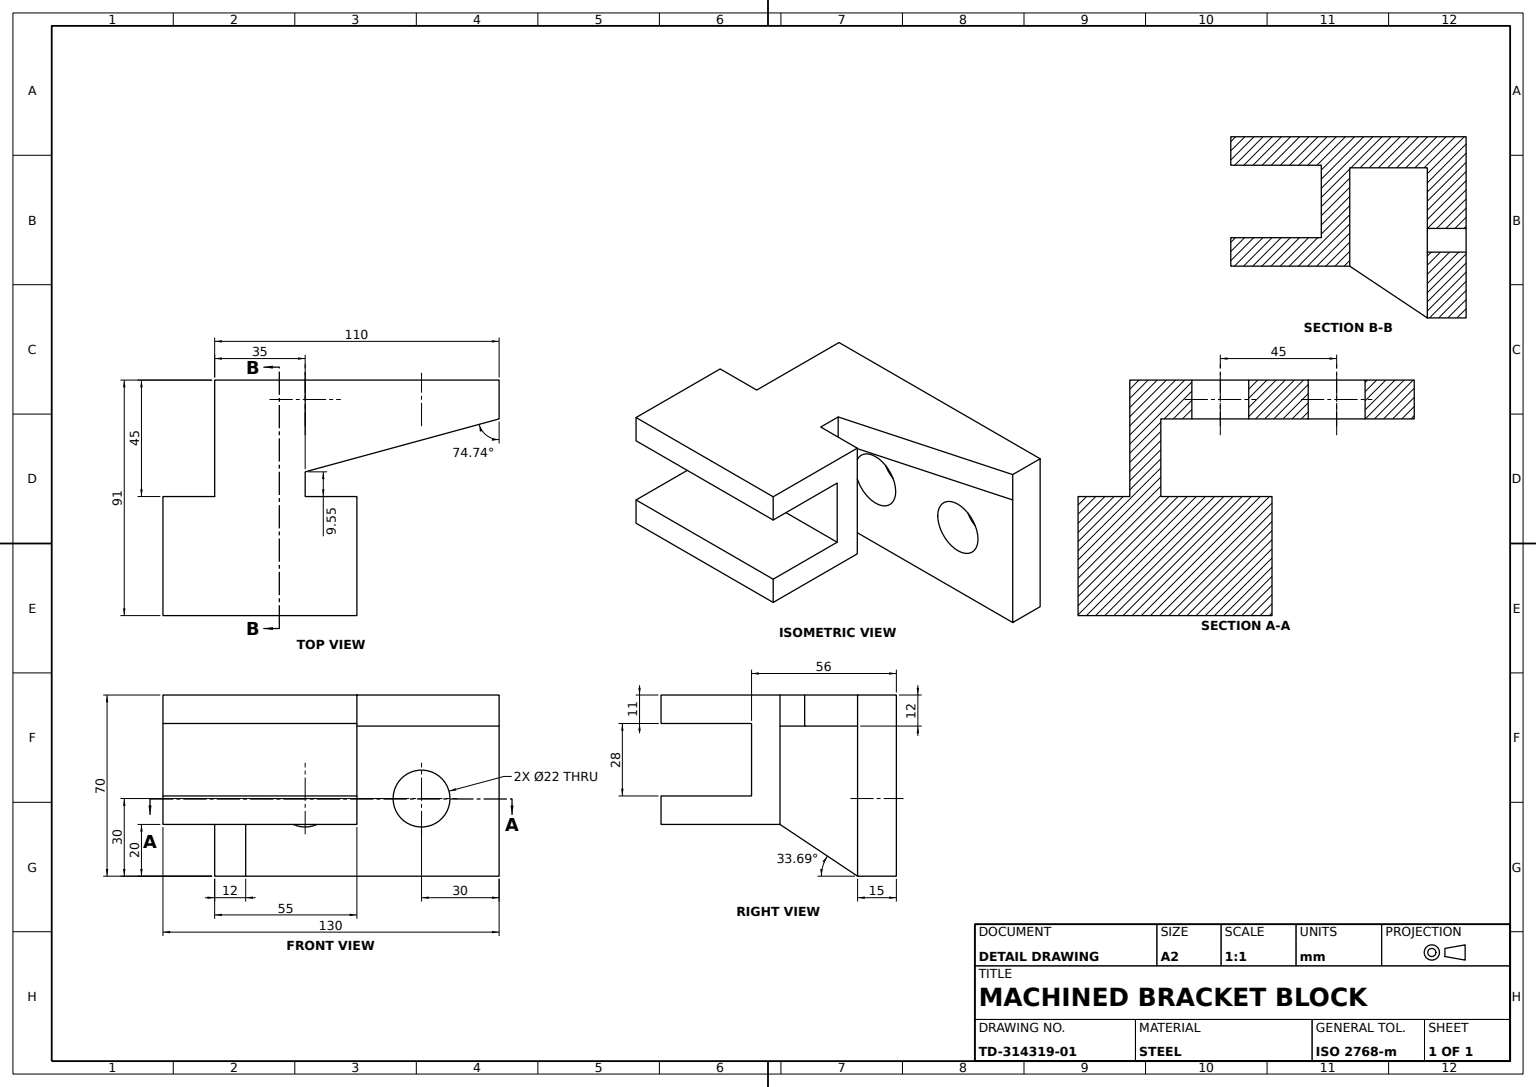
from build123d import *

# Parameters (mm, degrees)
BASE_PLATE_SKETCH_W         = 110
BASE_PLATE_SKETCH_H         = 70
BASE_PLATE_15MM_DEPTH       = 15
TRIANGULAR_WALL_12MM_DEPTH  = 12
WALL_EXTENSION_12MM_DEPTH   = 12
WEDGE_GUSSET_12MM_DEPTH     = 12
TOP_PROFILE_BOSS_11MM_DEPTH = 11
PROFILE_ARM_75MM_DEPTH      = 75
BLOCK_ARM_SKETCH_W          = 24
BLOCK_ARM_SKETCH_H          = 11
BLOCK_ARM_75MM_DEPTH        = 75
HOLE_CIRCLES_2X_22_SKETCH_R = 11
HOLES_2X_22_DEPTH           = 15
UPPER_JAW_SKETCH_W          = 11
UPPER_JAW_SKETCH_H          = 11
UPPER_JAW_75MM_DEPTH        = 75
LOWER_JAW_SKETCH_W          = 11
LOWER_JAW_SKETCH_H          = 11
LOWER_JAW_75MM_DEPTH        = 75


with BuildPart() as part:
    # Base Plate Sketch → Base Plate 15mm (new body)
    with BuildSketch(Plane.XY):
        with Locations((55, 35)):
            Rectangle(BASE_PLATE_SKETCH_W, BASE_PLATE_SKETCH_H)
    extrude(amount=BASE_PLATE_15MM_DEPTH)

    # Triangular Wall Sketch → Triangular Wall 12mm (add)
    with BuildSketch(Plane(origin=(0, 70, 0), x_dir=(1, 0, 0), z_dir=(0, 1, 0))):
        Polygon((0, -15), (0, -45), (110, -15), align=None)
    extrude(amount=-TRIANGULAR_WALL_12MM_DEPTH)

    # Wall Extension Sketch → Wall Extension 12mm (add)
    with BuildSketch(Plane.ZY):
        Polygon((45, 58), (45, 20), (15, 0), (15, 58), align=None)
    extrude(amount=-WALL_EXTENSION_12MM_DEPTH)

    # Wedge Gusset Sketch → Wedge Gusset 12mm (add)
    with BuildSketch(Plane(origin=(0, 70, 0), x_dir=(1, 0, 0), z_dir=(0, 1, 0))):
        Polygon((0, -45), (35, -45), (35, -35.454545455), align=None)
    extrude(amount=-WEDGE_GUSSET_12MM_DEPTH)

    # Top Profile Sketch → Top Profile Boss 11mm (add)
    with BuildSketch(Plane(origin=(0, 70, 0), x_dir=(1, 0, 0), z_dir=(0, 1, 0))):
        Polygon((17.5, -45), (55, -45), (55, -56), (-20, -56), (-20, -45), align=None)
    extrude(amount=-TOP_PROFILE_BOSS_11MM_DEPTH)

    # Profile Arm Sketch → Profile Arm 75mm (add)
    with BuildSketch(Plane(origin=(55, 0, 0), x_dir=(0, 0, -1), z_dir=(1, 0, 0))):
        Polygon((-45, 59), (-45, 31), (-45, 20), (-80, 20), (-80, 31), (-56, 31), (-56, 59), align=None)
    extrude(amount=-PROFILE_ARM_75MM_DEPTH)

    # Block Arm Sketch → Block Arm 75mm (add)
    with BuildSketch(Plane(origin=(55, 0, 0), x_dir=(0, 0, -1), z_dir=(1, 0, 0))):
        with Locations((-68, 64.5)):
            Rectangle(BLOCK_ARM_SKETCH_W, BLOCK_ARM_SKETCH_H)
    extrude(amount=-BLOCK_ARM_75MM_DEPTH)

    # Hole Circles 2xØ22 Sketch → Holes 2xØ22 (cut)
    with BuildSketch(Plane.XY.offset(15)):
        with Locations((80, 30)):
            Circle(HOLE_CIRCLES_2X_22_SKETCH_R)
        with Locations((35, 30)):
            Circle(HOLE_CIRCLES_2X_22_SKETCH_R)
    extrude(amount=-HOLES_2X_22_DEPTH, mode=Mode.SUBTRACT)

    # Upper Jaw Sketch → Upper Jaw 75mm (add)
    with BuildSketch(Plane(origin=(55, 0, 0), x_dir=(0, 0, -1), z_dir=(1, 0, 0))):
        with Locations((-85.5, 64.5)):
            Rectangle(UPPER_JAW_SKETCH_W, UPPER_JAW_SKETCH_H)
    extrude(amount=-UPPER_JAW_75MM_DEPTH)

    # Lower Jaw Sketch → Lower Jaw 75mm (add)
    with BuildSketch(Plane(origin=(55, 0, 0), x_dir=(0, 0, -1), z_dir=(1, 0, 0))):
        with Locations((-85.5, 25.5)):
            Rectangle(LOWER_JAW_SKETCH_W, LOWER_JAW_SKETCH_H)
    extrude(amount=-LOWER_JAW_75MM_DEPTH)


solid = part.part
